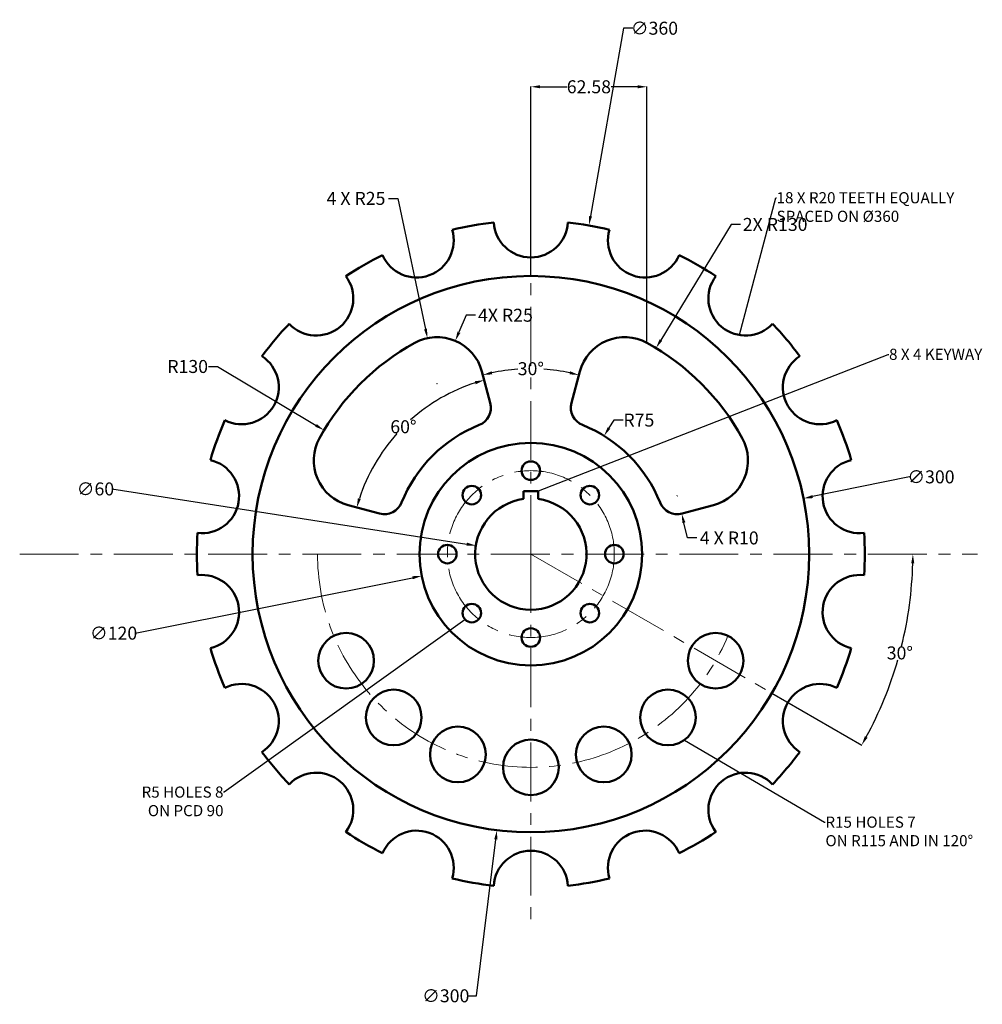
# Model space of a CAD drawing. Units: inches. Extents: x 288 to 807, y 153 to 684.
import ezdxf
from ezdxf import colors
from ezdxf.entities.mleader import LeaderData, LeaderLine
from ezdxf.math import Vec2, Vec3

# ---------------------------------------------------------------- set-up
doc = ezdxf.new("R2010")
doc.units = ezdxf.units.IN
doc.header["$MEASUREMENT"] = 0
doc.linetypes.add('CENTER', pattern=[50.8, 31.75, -6.35, 6.35, -6.35])
for name, color, linetype, lineweight in [('M-CNTR', 4, 'CENTER', 18), ('M-DIMS', 2, 'Continuous', 25), ('M-OUTL', 7, 'Continuous', 50), ('M-TEXT', 7, 'Continuous', 25)]:
    doc.layers.add(name, color=color, linetype=linetype, lineweight=lineweight)
doc.styles.get("Standard").update_dxf_attribs({"font": 'arial.ttf'})
doc.dimstyles.get("Standard").update_dxf_attribs({"dimtxt": 7, "dimasz": 5, "dimexe": 0.18, "dimexo": 0.0625, "dimgap": 0.09, "dimtad": 0, "dimtih": 1, "dimtoh": 1, "dimdec": 0, "dimzin": 0, "dimdsep": 46, "dimtxsty": 'Standard', "dimcen": 0.09, "dimclrd": 1, "dimclre": 1, "dimadec": 0, "dimazin": 0, "dimtfac": 1, "dimtdec": 0, "dimtofl": 0, "dimtmove": 0, "dimatfit": 3, "dimfxl": 1, "dimtolj": 1, "dimtzin": 0, "dimarcsym": 0})

# ---------------------------------------------------------------- blocks, each defined once
blk = doc.blocks.new('*U1')
blk.add_circle((0, 0), 5)
blk = doc.blocks.new('*U2')
at = {"layer": 'M-OUTL', "color": 0, "linetype": 'ByBlock', "lineweight": -2, "transparency": 16777216}
for p, rotation in [((563.73, 440.93), 90), ((531.91, 427.75), 135), ((595.55, 427.75), 45), ((518.73, 395.93), 180), ((531.91, 364.11), 225), ((595.55, 364.11), 315), ((563.73, 350.93), 270)]:
    blk.add_blockref('*U1', p, dxfattribs=dict(at, rotation=rotation))
blk.add_blockref('*U1', (608.73, 395.93), dxfattribs=at)
blk = doc.blocks.new('*U3')
blk.add_circle((0, 0), 15)
blk = doc.blocks.new('*U4')
at = {"layer": 'M-OUTL', "color": 0, "linetype": 'ByBlock', "lineweight": -2, "transparency": 16777216}
for p, rotation in [((464.14, 338.43), 240.0000000000002), ((489.81, 307.84), 260.0000000000002), ((637.66, 307.84), 340.0000000000001), ((603.07, 287.87), 320.0000000000001), ((524.4, 287.87), 280.0000000000001), ((563.73, 280.93), 300)]:
    blk.add_blockref('*U3', p, dxfattribs=dict(at, rotation=rotation))
blk.add_blockref('*U3', (663.33, 338.43), dxfattribs=at)
blk = doc.blocks.new('*D5')
at = {"layer": 'Defpoints', "color": 0, "transparency": 16777216}
for p in [(537.34, 494.44), (572.45, 495.55), (590.13, 494.44), (541.89, 477.47), (585.58, 477.47)]:
    blk.add_point(p, dxfattribs=at)
at = {"layer": 'M-DIMS', "color": 0, "lineweight": -2, "transparency": 16777216}
for start, end in [(93.9876, 102.1349), (77.8651, 86.0124)]:
    blk.add_arc((563.73, 395.93), 100, start, end, dxfattribs=at)
at = {"layer": 'M-DIMS', "color": 0, "transparency": 16777216}
for points in [[(542.91, 492.89), (542.52, 494.51), (537.85, 492.52)], [(584.95, 494.51), (584.56, 492.89), (589.62, 492.52)]]:
    blk.add_solid(points, dxfattribs=at)
at = {"layer": 'M-DIMS', "color": 0, "transparency": 16777216, "insert": (563.73, 495.93), "char_height": 7, "attachment_point": 5}
blk.add_mtext('\\A1;30°', dxfattribs=at)
blk = doc.blocks.new('*D6')
at = {"layer": 'Defpoints', "color": 0, "transparency": 16777216}
for p in [(603.22, 459.7), (563.73, 395.93)]:
    blk.add_point(p, dxfattribs=at)
at = {"layer": 'M-DIMS', "color": 0, "lineweight": -2, "transparency": 16777216}
for p, q in [((608.48, 468.2), (605.85, 463.95)), ((613.48, 468.2), (608.48, 468.2)), ((563.64, 395.93), (563.82, 395.93)), ((563.73, 395.84), (563.73, 396.02))]:
    blk.add_line(p, q, dxfattribs=at)
at = {"layer": 'M-DIMS', "color": 0, "transparency": 16777216}
blk.add_solid([(605.14, 464.39), (606.56, 463.51), (603.22, 459.7)], dxfattribs=at)
at = {"layer": 'M-DIMS', "color": 0, "transparency": 16777216, "insert": (621.96, 468.2), "char_height": 7, "attachment_point": 5}
blk.add_mtext('\\A1;R75', dxfattribs=at)
blk = doc.blocks.new('*D7')
at = {"layer": 'Defpoints', "color": 0, "transparency": 16777216}
for p in [(537.34, 494.44), (508.01, 475.52), (541.89, 477.47), (465.23, 422.33), (482.2, 417.78)]:
    blk.add_point(p, dxfattribs=at)
at = {"layer": 'M-DIMS', "color": 0, "lineweight": -2, "transparency": 16777216}
for start, end in [(107.9491, 131.8563), (137.9798, 162.0509)]:
    blk.add_arc((563.73, 395.93), 97.15, start, end, dxfattribs=at)
at = {"layer": 'M-DIMS', "color": 0, "transparency": 16777216}
for points in [[(533.56, 489.16), (534.03, 487.56), (538.59, 489.78)], [(472.11, 425.64), (470.51, 426.11), (469.89, 421.08)]]:
    blk.add_solid(points, dxfattribs=at)
at = {"layer": 'M-DIMS', "color": 0, "transparency": 16777216, "insert": (495.04, 464.63), "char_height": 7, "attachment_point": 5}
blk.add_mtext('\\A1;60°', dxfattribs=at)
blk = doc.blocks.new('*U8')
blk.add_arc((0, 10.56), 20, 183.1847, 356.8153)
blk = doc.blocks.new('*U9')
at = {"layer": 'M-OUTL', "color": 0, "linetype": 'ByBlock', "lineweight": -2, "transparency": 16777216}
blk.add_blockref('*U8', (563.73, 565.38), dxfattribs=at)
for p, rotation in [((505.78, 555.16), 19.99999999999997), ((621.69, 555.16), 339.9999999999999), ((454.82, 525.74), 39.99999999999999), ((672.65, 525.74), 320), ((416.99, 480.66), 59.99999999999999), ((710.48, 480.66), 300), ((396.86, 425.36), 79.99999999999999), ((730.6, 425.36), 280), ((396.86, 366.51), 99.99999999999996), ((730.6, 366.51), 260), ((416.99, 311.21), 120), ((710.48, 311.21), 239.9999999999999), ((454.82, 266.13), 140), ((672.65, 266.13), 219.9999999999999), ((505.78, 236.71), 160), ((621.69, 236.71), 199.9999999999999), ((563.73, 226.49), 180)]:
    blk.add_blockref('*U8', p, dxfattribs=dict(at, rotation=rotation))
blk = doc.blocks.new('*D10')
at = {"layer": 'Defpoints', "color": 0, "transparency": 16777216}
for p in [(507.99, 512.42), (513.19, 487.97)]:
    blk.add_point(p, dxfattribs=at)
at = {"layer": 'M-DIMS', "color": 0, "lineweight": -2, "transparency": 16777216}
for p, q in [((486.98, 587.78), (491.98, 587.78)), ((491.98, 587.78), (506.95, 517.31)), ((513.1, 487.97), (513.28, 487.97)), ((513.19, 487.88), (513.19, 488.06))]:
    blk.add_line(p, q, dxfattribs=at)
at = {"layer": 'M-DIMS', "color": 0, "transparency": 16777216}
blk.add_solid([(507.77, 517.49), (506.14, 517.14), (507.99, 512.42)], dxfattribs=at)
at = {"layer": 'M-DIMS', "color": 0, "transparency": 16777216, "insert": (469.48, 587.78), "char_height": 7, "attachment_point": 5}
blk.add_mtext('\\A1;4 X R25', dxfattribs=at)
blk = doc.blocks.new('*D11')
at = {"layer": 'Defpoints', "color": 0, "transparency": 16777216}
for p in [(452.23, 462.76), (563.73, 395.93)]:
    blk.add_point(p, dxfattribs=at)
at = {"layer": 'M-DIMS', "color": 0, "lineweight": -2, "transparency": 16777216}
for p, q in [((389.9, 497.12), (394.9, 497.12)), ((394.9, 497.12), (447.94, 465.33)), ((563.64, 395.93), (563.82, 395.93)), ((563.73, 395.84), (563.73, 396.02))]:
    blk.add_line(p, q, dxfattribs=at)
at = {"layer": 'M-DIMS', "color": 0, "transparency": 16777216}
blk.add_solid([(448.37, 466.05), (447.51, 464.62), (452.23, 462.76)], dxfattribs=at)
at = {"layer": 'M-DIMS', "color": 0, "transparency": 16777216, "insert": (378.74, 497.12), "char_height": 7, "attachment_point": 5}
blk.add_mtext('\\A1;R130', dxfattribs=at)
blk = doc.blocks.new('*D12')
at = {"layer": 'Defpoints', "color": 0, "transparency": 16777216}
for p in [(534.09, 400.55), (593.38, 391.32)]:
    blk.add_point(p, dxfattribs=at)
at = {"layer": 'M-DIMS', "color": 0, "lineweight": -2, "transparency": 16777216}
for p, q in [((337.94, 431.09), (529.15, 401.32)), ((563.64, 395.93), (563.82, 395.93)), ((563.73, 395.84), (563.73, 396.02))]:
    blk.add_line(p, q, dxfattribs=at)
at = {"layer": 'M-DIMS', "color": 0, "transparency": 16777216}
blk.add_solid([(529.28, 402.14), (529.02, 400.49), (534.09, 400.55)], dxfattribs=at)
at = {"layer": 'M-DIMS', "color": 0, "transparency": 16777216, "insert": (329.04, 431.09), "char_height": 7, "attachment_point": 5}
blk.add_mtext('\\A1;∅60', dxfattribs=at)
blk = doc.blocks.new('*D13')
at = {"layer": 'Defpoints', "color": 0, "transparency": 16777216}
for p in [(622.57, 407.69), (504.9, 384.17)]:
    blk.add_point(p, dxfattribs=at)
at = {"layer": 'M-DIMS', "color": 0, "lineweight": -2, "transparency": 16777216}
for p, q in [((563.64, 395.93), (563.82, 395.93)), ((563.73, 395.84), (563.73, 396.02)), ((350.44, 353.3), (500, 383.19))]:
    blk.add_line(p, q, dxfattribs=at)
at = {"layer": 'M-DIMS', "color": 0, "transparency": 16777216}
blk.add_solid([(499.83, 384.01), (500.16, 382.38), (504.9, 384.17)], dxfattribs=at)
at = {"layer": 'M-DIMS', "color": 0, "transparency": 16777216, "insert": (338.82, 353.3), "char_height": 7, "attachment_point": 5}
blk.add_mtext('\\A1;∅120', dxfattribs=at)
blk = doc.blocks.new('*D14')
at = {"layer": 'Defpoints', "color": 0, "transparency": 16777216}
for p in [(642.68, 427.44), (645.05, 417.72)]:
    blk.add_point(p, dxfattribs=at)
at = {"layer": 'M-DIMS', "color": 0, "lineweight": -2, "transparency": 16777216}
for p, q in [((642.59, 427.44), (642.77, 427.44)), ((642.68, 427.35), (642.68, 427.53)), ((648.23, 404.65), (646.23, 412.87)), ((653.23, 404.65), (648.23, 404.65))]:
    blk.add_line(p, q, dxfattribs=at)
at = {"layer": 'M-DIMS', "color": 0, "transparency": 16777216}
blk.add_solid([(647.04, 413.06), (645.42, 412.67), (645.05, 417.72)], dxfattribs=at)
at = {"layer": 'M-DIMS', "color": 0, "transparency": 16777216, "insert": (670.69, 404.65), "char_height": 7, "attachment_point": 5}
blk.add_mtext('\\A1;4 X R10', dxfattribs=at)
blk = doc.blocks.new('*D15')
at = {"layer": 'Defpoints', "color": 0, "transparency": 16777216}
for p in [(710.7, 425.93), (416.76, 365.93)]:
    blk.add_point(p, dxfattribs=at)
at = {"layer": 'M-DIMS', "color": 0, "lineweight": -2, "transparency": 16777216}
for p, q in [((767.8, 437.59), (715.6, 426.93)), ((563.64, 395.93), (563.82, 395.93)), ((563.73, 395.84), (563.73, 396.02))]:
    blk.add_line(p, q, dxfattribs=at)
at = {"layer": 'M-DIMS', "color": 0, "transparency": 16777216}
blk.add_solid([(715.44, 427.75), (715.77, 426.12), (710.7, 425.93)], dxfattribs=at)
at = {"layer": 'M-DIMS', "color": 0, "transparency": 16777216, "insert": (779.42, 437.59), "char_height": 7, "attachment_point": 5}
blk.add_mtext('\\A1;∅300', dxfattribs=at)
blk = doc.blocks.new('*D16')
at = {"layer": 'Defpoints', "color": 0, "transparency": 16777216}
for p in [(288.2, 395.93), (563.73, 395.93), (804.54, 395.93), (757.24, 325.5), (693.64, 320.93)]:
    blk.add_point(p, dxfattribs=at)
at = {"layer": 'M-DIMS', "color": 0, "lineweight": -2, "transparency": 16777216}
blk.add_line((693.69, 320.9), (742.23, 292.88), dxfattribs=at)
for start, end in [(346.0536, 358.6088), (331.3912, 343.9412)]:
    blk.add_arc((563.73, 395.93), 205.92, start, end, dxfattribs=at)
at = {"layer": 'M-DIMS', "color": 0, "transparency": 16777216}
for points in [[(768.76, 390.94), (770.43, 390.92), (769.66, 395.93)], [(745.24, 296.92), (743.79, 297.74), (742.07, 292.97)]]:
    blk.add_solid(points, dxfattribs=at)
at = {"layer": 'M-DIMS', "color": 0, "transparency": 16777216, "insert": (762.64, 342.64), "char_height": 7, "attachment_point": 5}
blk.add_mtext('\\A1;30°', dxfattribs=at)
blk = doc.blocks.new('SPROCKET-WEB-SLOT')
for p, q in [((0.34, 60.03), (4.89, 77)), ((60.03, 0.34), (77, 4.89))]:
    blk.add_line(p, q)
for centre, radius, start, end in [((29.04, 70.53), 25, 61.2259, 165), ((-21.51, -21.51), 130, 28.7741, 61.2259), ((10, 57.44), 10, 165, 248.2437), ((-21.51, -21.51), 75, 21.7563, 68.2437), ((70.53, 29.04), 25, 285, 28.7741), ((57.44, 10), 10, 201.7563, 285)]:
    blk.add_arc(centre, radius, start, end)
blk = doc.blocks.new('*D18')
at = {"layer": 'Defpoints', "color": 0, "transparency": 16777216}
for p in [(626.31, 647.97), (563.73, 545.93), (626.31, 509.88)]:
    blk.add_point(p, dxfattribs=at)
at = {"layer": 'M-DIMS', "color": 1, "lineweight": -2, "transparency": 16777216}
for p, q in [((563.73, 546), (563.73, 648.15)), ((568.73, 647.97), (583.1, 647.97)), ((621.31, 647.97), (606.95, 647.97)), ((626.31, 509.94), (626.31, 648.15))]:
    blk.add_line(p, q, dxfattribs=at)
at = {"layer": 'M-DIMS', "color": 1, "transparency": 16777216}
for points in [[(568.73, 648.81), (568.73, 647.14), (563.73, 647.97)], [(621.31, 648.81), (621.31, 647.14), (626.31, 647.97)]]:
    blk.add_solid(points, dxfattribs=at)
at = {"layer": 'M-DIMS', "color": 0, "transparency": 16777216, "insert": (595.02, 647.97), "char_height": 7, "attachment_point": 5}
blk.add_mtext('\\A1;62.58', dxfattribs=at)
blk = doc.blocks.new('*D19')
at = {"layer": 'Defpoints', "color": 0, "transparency": 16777216}
for p in [(594.99, 573.2), (532.48, 218.67)]:
    blk.add_point(p, dxfattribs=at)
at = {"layer": 'M-DIMS', "color": 1, "lineweight": -2, "transparency": 16777216}
for p, q in [((613.74, 679.56), (595.86, 578.12)), ((618.74, 679.56), (613.74, 679.56)), ((563.64, 395.93), (563.82, 395.93)), ((563.73, 395.84), (563.73, 396.02))]:
    blk.add_line(p, q, dxfattribs=at)
at = {"layer": 'M-DIMS', "color": 1, "transparency": 16777216}
blk.add_solid([(595.04, 578.27), (596.68, 577.98), (594.99, 573.2)], dxfattribs=at)
at = {"layer": 'M-DIMS', "color": 0, "transparency": 16777216, "insert": (630.36, 679.56), "char_height": 7, "attachment_point": 5}
blk.add_mtext('\\A1;∅360', dxfattribs=at)
blk = doc.blocks.new('*D20')
at = {"layer": 'Defpoints', "color": 0, "transparency": 16777216}
for p in [(582.02, 544.81), (545.45, 247.05)]:
    blk.add_point(p, dxfattribs=at)
at = {"layer": 'M-DIMS', "color": 1, "lineweight": -2, "transparency": 16777216}
for p, q in [((563.64, 395.93), (563.82, 395.93)), ((563.73, 395.84), (563.73, 396.02)), ((534.48, 157.72), (544.84, 242.09)), ((529.48, 157.72), (534.48, 157.72))]:
    blk.add_line(p, q, dxfattribs=at)
at = {"layer": 'M-DIMS', "color": 1, "transparency": 16777216}
blk.add_solid([(544.01, 242.19), (545.67, 241.99), (545.45, 247.05)], dxfattribs=at)
at = {"layer": 'M-DIMS', "color": 0, "transparency": 16777216, "insert": (517.86, 157.72), "char_height": 7, "attachment_point": 5}
blk.add_mtext('\\A1;∅300', dxfattribs=at)
blk = doc.blocks.new('*D21')
at = {"layer": 'Defpoints', "color": 0, "transparency": 16777216}
for p in [(631.2, 507.05), (563.73, 395.93)]:
    blk.add_point(p, dxfattribs=at)
at = {"layer": 'M-DIMS', "color": 1, "lineweight": -2, "transparency": 16777216}
for p, q in [((671.68, 573.73), (633.8, 511.33)), ((676.68, 573.73), (671.68, 573.73)), ((563.64, 395.93), (563.82, 395.93)), ((563.73, 395.84), (563.73, 396.02))]:
    blk.add_line(p, q, dxfattribs=at)
at = {"layer": 'M-DIMS', "color": 1, "transparency": 16777216}
blk.add_solid([(633.09, 511.76), (634.51, 510.9), (631.2, 507.05)], dxfattribs=at)
at = {"layer": 'M-DIMS', "color": 0, "transparency": 16777216, "insert": (695.42, 573.73), "char_height": 7, "attachment_point": 5}
blk.add_mtext('\\A1;2X R130', dxfattribs=at)
blk = doc.blocks.new('*D22')
at = {"layer": 'Defpoints', "color": 0, "transparency": 16777216}
for p in [(523.01, 510.96), (513.19, 487.97)]:
    blk.add_point(p, dxfattribs=at)
at = {"layer": 'M-DIMS', "color": 1, "lineweight": -2, "transparency": 16777216}
for p, q in [((528.89, 524.76), (524.97, 515.56)), ((533.89, 524.76), (528.89, 524.76)), ((513.1, 487.97), (513.28, 487.97)), ((513.19, 487.88), (513.19, 488.06))]:
    blk.add_line(p, q, dxfattribs=at)
at = {"layer": 'M-DIMS', "color": 1, "transparency": 16777216}
blk.add_solid([(524.2, 515.89), (525.74, 515.23), (523.01, 510.96)], dxfattribs=at)
at = {"layer": 'M-DIMS', "color": 0, "transparency": 16777216, "insert": (550.03, 524.76), "char_height": 7, "attachment_point": 5}
blk.add_mtext('\\A1;4X R25', dxfattribs=at)

msp = doc.modelspace()

# ---------------------------------------------------------------- linework, layer by layer
at = {"layer": 'M-CNTR'}
for p, q in [((563.735, 395.933), (563.735, 621.524)), ((288.205, 395.933), (804.542, 395.933)), ((563.735, 395.933), (693.638, 320.933)), ((563.735, 395.933), (563.735, 198.391))]:
    msp.add_line(p, q, dxfattribs=at)
msp.add_circle((563.735, 395.933), 45, dxfattribs=at)
msp.add_arc((563.735, 395.933), 115, 180, 337.47867, dxfattribs=at)
at = {"layer": 'M-OUTL'}
for p, q in [((559.735, 429.933), (567.735, 429.933)), ((559.735, 429.933), (559.735, 425.665)), ((567.735, 429.933), (567.735, 425.665))]:
    msp.add_line(p, q, dxfattribs=at)
for radius in [150, 60]:
    msp.add_circle((563.735, 395.933), radius, dxfattribs=at)
for radius, start, end in [(180, 96.36948, 103.63052), (180, 76.36948, 83.63052), (180, 116.36948, 123.63052), (180, 56.36948, 63.63052), (180, 136.36948, 143.63052), (180, 36.36948, 43.63052), (180, 156.36948, 163.63052), (180, 16.36948, 23.63052), (30, 97.66226, 82.33774), (180, 176.36948, 183.63052), (180, 356.36948, 3.63052), (180, 196.36948, 203.63052), (180, 336.36948, 343.63052), (180, 216.36948, 223.63052), (180, 316.36948, 323.63052), (180, 236.36948, 243.63052), (180, 296.36948, 303.63052), (180, 256.36948, 263.63052), (180, 276.36948, 283.63052)]:
    msp.add_arc((563.735, 395.933), radius, start, end, dxfattribs=at)

# ---------------------------------------------------------------- block references
for name, p in [('*U9', (0, 0)), ('SPROCKET-WEB-SLOT', (585.24, 417.439)), ('*U2', (0, 0)), ('*U4', (0, 0))]:
    msp.add_blockref(name, p, dxfattribs=at)
at = {"layer": 'M-OUTL', "rotation": 89.99999999999999}
msp.add_blockref('SPROCKET-WEB-SLOT', (542.229, 417.439), dxfattribs=at)

# ---------------------------------------------------------------- dimensions: what is measured, and where the dimension line sits
at = {"layer": 'M-DIMS'}
for p1, p2, override, picture, middle in [((532.478, 218.668), (594.991, 573.199), {"dimdec": 0, "dimlfac": 1, "dimrnd": 0, "dimzin": 0, "dimdsep": 46, "dimlunit": 2}, '*D19', (630.364, 679.558)), ((582.019, 544.815), (545.45, 247.052), {"dimdec": 0, "dimlfac": 1, "dimrnd": 0, "dimzin": 0, "dimdsep": 46, "dimlunit": 2}, '*D20', (517.861, 157.723)), ((416.765, 365.935), (710.704, 425.932), {"dimclrd": 0, "dimclre": 0, "dimclrt": 0}, '*D15', (767.803, 437.587)), ((593.377, 391.318), (534.092, 400.549), {"dimclrd": 0, "dimclre": 0, "dimclrt": 0}, '*D12', (337.938, 431.092)), ((622.571, 407.693), (504.898, 384.174), {"dimclrd": 0, "dimclre": 0, "dimclrt": 0}, '*D13', (350.439, 353.302))]:
    dim = msp.add_diameter_dim_2p(p1=p1, p2=p2, dimstyle='Standard', override=override, dxfattribs=at)
    dim.commit()
    dim.dimension.update_dxf_attribs({"geometry": picture, "text_midpoint": middle, "dimtype": 163})
dim = msp.add_linear_dim(base=(626.311, 647.974), p1=(563.735, 545.933), p2=(626.311, 509.881), dimstyle='Standard', override={"dimdec": 2, "dimlfac": 1, "dimrnd": 0, "dimzin": 0, "dimdsep": 46, "dimlunit": 2}, dxfattribs=at)
dim.commit()
dim.dimension.update_dxf_attribs({"geometry": '*D18', "text_midpoint": (595.023, 647.974)})
for center, mpoint, text, override, picture, middle in [((513.192, 487.968), (507.994, 512.422), '4 X <>', {"dimclrd": 0, "dimclre": 0, "dimclrt": 0}, '*D10', (469.477, 587.778)), ((563.735, 395.933), (631.203, 507.055), '2X <>', {"dimdec": 0, "dimlfac": 1, "dimrnd": 0, "dimzin": 0, "dimdsep": 46, "dimlunit": 2}, '*D21', (695.425, 573.728)), ((513.192, 487.968), (523.006, 510.962), '4X <>', {"dimdec": 0, "dimlfac": 1, "dimrnd": 0, "dimzin": 0, "dimdsep": 46, "dimlunit": 2}, '*D22', (550.035, 524.757)), ((642.68, 427.439), (645.047, 417.724), '4 X <>', {"dimclrd": 0, "dimclre": 0, "dimclrt": 0}, '*D14', (670.694, 404.65))]:
    dim = msp.add_radius_dim(center=center, mpoint=mpoint, text=text, dimstyle='Standard', override=override, dxfattribs=at)
    dim.commit()
    dim.dimension.update_dxf_attribs({"geometry": picture, "text_midpoint": middle, "dimtype": 164})
dim = msp.add_radius_dim(center=(563.735, 395.933), mpoint=(452.227, 462.761), dimstyle='Standard', override={"dimclrd": 0, "dimclre": 0, "dimclrt": 0}, dxfattribs=at)
dim.commit()
dim.dimension.update_dxf_attribs({"geometry": '*D11', "text_midpoint": (378.737, 497.119), "dimtype": 164})
for base, line1, line2, picture, middle in [((572.45, 495.552), ((585.581, 477.467), (590.129, 494.439)), ((541.888, 477.467), (537.34, 494.439)), '*D5', (563.735, 495.932)), ((508.01, 475.516), ((541.888, 477.467), (537.34, 494.439)), ((482.201, 417.78), (465.229, 422.328)), '*D7', (495.037, 464.631)), ((757.239, 325.503), ((288.205, 395.933), (804.542, 395.933)), ((563.735, 395.933), (693.638, 320.933)), '*D16', (762.641, 342.636))]:
    dim = msp.add_angular_dim_2l(base=base, line1=line1, line2=line2, dimstyle='Standard', override={"dimclrd": 0, "dimclre": 0, "dimclrt": 0}, dxfattribs=at)
    dim.commit()
    dim.dimension.update_dxf_attribs({"geometry": picture, "text_midpoint": middle})
dim = msp.add_radius_dim(center=(563.735, 395.933), mpoint=(603.218, 459.699), dimstyle='Standard', override={"dimclrd": 0, "dimclre": 0, "dimclrt": 0}, dxfattribs=at)
dim.commit()
dim.dimension.update_dxf_attribs({"geometry": '*D6', "text_midpoint": (621.962, 468.201)})

# ---------------------------------------------------------------- leaders
at = {"layer": 'M-TEXT'}
ml = msp.add_multileader_mtext('Standard', dxfattribs=at)
ml.set_content('18 X R20 TEETH EQUALLY \\PSPACED ON %%C360', color=256)
ml.set_leader_properties()
ml.build(insert=Vec2(0, 0))
ml.multileader.update_dxf_attribs({"dogleg_length": 0.36, "arrow_head_size": 0.18})
ctx = ml.context
ctx.base_point, ctx.char_height, ctx.arrow_head_size, ctx.landing_gap_size, ctx.plane_origin = Vec3(696.108, 588.004), 6, 0.18, 0.09, Vec3(676.18, 514.088)
notes = []
notes.append((ctx, [(0, (1, 1, 0), (695.748, 588.004), (1, 0), 0.36, [(0, [(676.18, 514.088)], 0, [])])]))
ctx.mtext.insert, ctx.mtext.flow_direction = Vec3(696.198, 591.124), 5
ml = msp.add_multileader_mtext('Standard', dxfattribs=at)
ml.set_content('8 X 4 KEYWAY', color=256)
ml.set_leader_properties()
ml.build(insert=Vec2(0, 0))
ml.multileader.update_dxf_attribs({"dogleg_length": 0.36, "arrow_head_size": 0.18})
ctx = ml.context
ctx.base_point, ctx.char_height, ctx.arrow_head_size, ctx.landing_gap_size, ctx.plane_origin = Vec3(756.742, 503.633), 6, 0.18, 0.09, Vec3(567.735, 429.933)
notes.append((ctx, [(0, (1, 1, 0), (756.382, 503.633), (1, 0), 0.36, [(0, [(567.735, 429.933)], 0, [])])]))
ctx.mtext.insert, ctx.mtext.flow_direction = Vec3(756.832, 506.684), 5
ml = msp.add_multileader_mtext('Standard', dxfattribs=at)
ml.set_content('R5 HOLES 8\\PON PCD 90', color=256)
ml.set_leader_properties()
ml.build(insert=Vec2(0, 0))
ml.multileader.update_dxf_attribs({"dogleg_length": 0.36, "arrow_head_size": 0.18})
ctx = ml.context
ctx.base_point, ctx.char_height, ctx.arrow_head_size, ctx.landing_gap_size, ctx.plane_origin = Vec3(350.535, 267.533), 6, 0.18, 0.09, Vec3(528.379, 360.578)
ctx.text_align_type = 2
notes.append((ctx, [(0, (1, 1, 0), (398.498, 267.533), (-1, 0), 0.36, [(0, [(528.379, 360.578)], 0, [])])]))
ctx.mtext.insert, ctx.mtext.alignment, ctx.mtext.flow_direction = Vec3(398.048, 270.584), 3, 5
ml = msp.add_multileader_mtext('Standard', dxfattribs=at)
ml.set_content('R15 HOLES 7 \\PON R115 AND IN 120°', color=256)
ml.set_leader_properties()
ml.build(insert=Vec2(0, 0))
ml.multileader.update_dxf_attribs({"dogleg_length": 0.36, "arrow_head_size": 0.18})
ctx = ml.context
ctx.base_point, ctx.char_height, ctx.arrow_head_size, ctx.landing_gap_size, ctx.plane_origin = Vec3(722.426, 251.321), 6, 0.18, 0.09, Vec3(646.374, 295.632)
notes.append((ctx, [(0, (1, 1, 0), (722.066, 251.321), (1, 0), 0.36, [(0, [(646.374, 295.632)], 0, [])])]))
ctx.mtext.insert, ctx.mtext.flow_direction = Vec3(722.516, 254.372), 5
for ctx, leaders in notes:
    for number, flags, end, landing, length, lines in leaders:
        leader = LeaderData()
        leader.index, (leader.has_last_leader_line, leader.has_dogleg_vector, leader.attachment_direction) = number, flags
        leader.last_leader_point, leader.dogleg_vector, leader.dogleg_length = Vec3(end), Vec3(landing), length
        for number, points, colour, breaks in lines:
            line = LeaderLine()
            line.index, line.vertices, line.color, line.breaks = number, Vec3.list(points), colors.encode_raw_color(colour), breaks
            leader.lines.append(line)
        ctx.leaders.append(leader)

doc.saveas('drawing.dxf')
